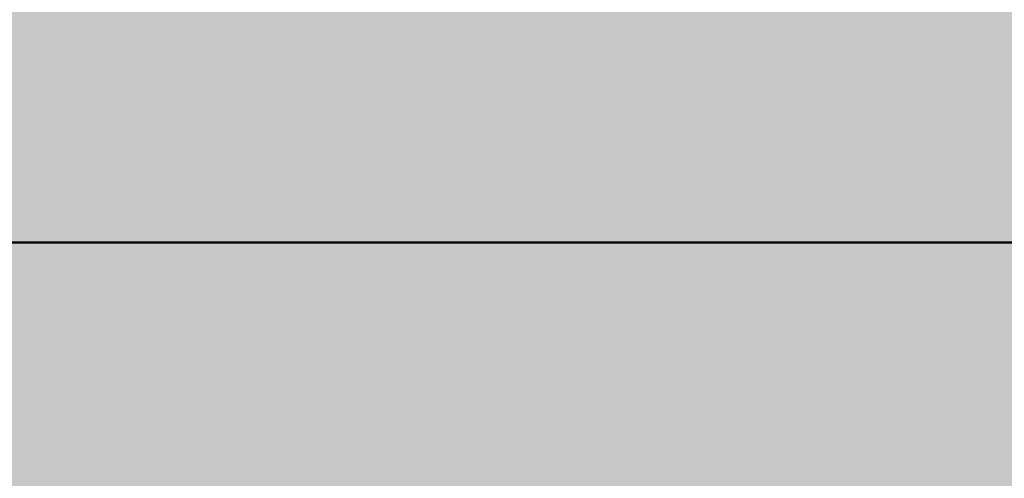
# Model space of a CAD drawing. Units: millimetres. Extents: x 0 to 2267, y 0 to 1823.
# Tile 142 of 256: x 1802 to 1823, y 1122 to 1132. Entities that reach past the tile are written whole.
import ezdxf

# ---------------------------------------------------------------- set-up
doc = ezdxf.new("R2010")
doc.units = ezdxf.units.MM
doc.header["$MEASUREMENT"] = 0
for name, color, linetype, lineweight in [('M-DIMS', 2, 'Continuous', 25), ('M-HATC', 252, 'Continuous', 18), ('M-OUTL', 7, 'Continuous', 50)]:
    doc.layers.add(name, color=color, linetype=linetype, lineweight=lineweight)
doc.styles.get("Standard").update_dxf_attribs({"font": 'arial.ttf'})
doc.dimstyles.get("Standard").update_dxf_attribs({"dimtxt": 7, "dimasz": 4, "dimexe": 0.18, "dimexo": 0.0625, "dimgap": 0.09, "dimtad": 0, "dimdec": 0, "dimzin": 0, "dimdsep": 46, "dimtxsty": 'Standard', "dimcen": 0.09, "dimadec": 0, "dimazin": 0, "dimtfac": 1, "dimtdec": 0, "dimtofl": 0, "dimtmove": 0, "dimatfit": 3, "dimfxl": 1, "dimtolj": 1, "dimtzin": 0, "dimarcsym": 0})

# ---------------------------------------------------------------- blocks, each defined once
blk = doc.blocks.new('*D1')
at = {"layer": 'Defpoints', "color": 0, "transparency": 16777216}
for p in [(1593.429, 1127.417), (1843.429, 1127.417), (1843.429, 955.628)]:
    blk.add_point(p, dxfattribs=at)
at = {"layer": 'M-DIMS', "color": 0, "lineweight": -2, "transparency": 16777216}
for p, q in [((1593.429, 1127.355), (1593.429, 955.448)), ((1843.429, 1127.355), (1843.429, 955.448)), ((1597.429, 955.628), (1710.558, 955.628)), ((1839.429, 955.628), (1726.3, 955.628))]:
    blk.add_line(p, q, dxfattribs=at)
at = {"layer": 'M-DIMS', "color": 0, "transparency": 16777216}
for points in [[(1597.429, 956.294), (1597.429, 954.961), (1593.429, 955.628)], [(1839.429, 956.294), (1839.429, 954.961), (1843.429, 955.628)]]:
    blk.add_solid(points, dxfattribs=at)
at = {"layer": 'M-DIMS', "color": 0, "transparency": 16777216, "insert": (1718.429, 955.628), "char_height": 7, "attachment_point": 5}
blk.add_mtext('\\A1;250', dxfattribs=at)

msp = doc.modelspace()

# ---------------------------------------------------------------- hatches: boundary and pattern name
at = {"layer": 'M-HATC'}
h = msp.add_hatch(color=256, dxfattribs=at)
h.dxf.hatch_style = 1
h.paths.add_polyline_path([(2055.771, 1603.062), (1381.087, 1603.062), (1381.087, 1598.062), (2055.771, 1598.062)])
h.paths.add_polyline_path([(2055.771, 1598.062), (1381.087, 1598.062), (1381.087, 1593.062), (2055.771, 1593.062)])
h.paths.add_polyline_path([(2051.307, 1536.761), (1385.55, 1536.761), (1385.55, 1526.761), (1387.55, 1526.761), (1388.537, 1525.053), (1385.332, 1521.233), (1385.332, 1521.223), (2050.254, 1522.749), (2048.321, 1525.053), (2049.307, 1526.761), (2051.307, 1526.761)])
edge = h.paths.add_edge_path()
edge.add_arc((1847.535, 1379.149), 135, 222.60306, 222.89085, ccw=False)
edge.add_line((1748.166, 1287.766), (1683.092, 1287.766))
edge.add_arc((1583.724, 1379.149), 135, 317.10915, 317.39694, ccw=False)
edge.add_arc((1678.969, 1290.671), 5, 222.8909, 317.1091, ccw=False)
edge.add_arc((1774.213, 1379.149), 135, 222.60306, 222.89085, ccw=False)
edge.add_line((1674.845, 1287.766), (1609.771, 1287.766))
edge.add_arc((1510.403, 1379.149), 135, 317.10915, 317.39694, ccw=False)
edge.add_arc((1605.647, 1290.671), 5, 222.8909, 317.1091, ccw=False)
edge.add_arc((1700.892, 1379.149), 135, 222.60306, 222.89085, ccw=False)
edge.add_line((1601.524, 1287.766), (1536.45, 1287.766))
edge.add_arc((1437.081, 1379.149), 135, 317.10915, 317.39694, ccw=False)
edge.add_arc((1532.326, 1290.671), 5, 222.8909, 317.1091, ccw=False)
edge.add_arc((1627.571, 1379.149), 135, 222.60306, 222.89085, ccw=False)
edge.add_line((1528.203, 1287.766), (1505.929, 1287.766))
edge.add_spline(control_points=[(1505.929, 1287.766), (1504.262, 1287.766), (1504.262, 1282.766), (1505.929, 1282.766)], knot_values=[0, 0, 0, 0, 5, 5, 5, 5], degree=3, periodic=0)
edge.add_line((1505.929, 1282.766), (1930.929, 1282.766))
edge.add_spline(control_points=[(1930.929, 1282.766), (1932.596, 1282.766), (1932.596, 1287.766), (1930.929, 1287.766)], knot_values=[0, 0, 0, 0, 5, 5, 5, 5], degree=3, periodic=0)
edge.add_line((1930.929, 1287.766), (1903.056, 1287.766))
edge.add_arc((1803.688, 1379.149), 135, 317.10915, 317.39694, ccw=False)
edge.add_arc((1898.932, 1290.671), 5, 222.8909, 317.1091, ccw=False)
edge.add_arc((1994.177, 1379.149), 135, 222.60306, 222.89085, ccw=False)
edge.add_line((1894.809, 1287.766), (1829.735, 1287.766))
edge.add_arc((1730.366, 1379.149), 135, 317.10915, 317.39694, ccw=False)
edge.add_arc((1825.611, 1290.671), 5, 222.8909, 317.1091, ccw=False)
edge.add_arc((1920.856, 1379.149), 135, 222.60306, 222.89085, ccw=False)
edge.add_line((1821.487, 1287.766), (1756.413, 1287.766))
edge.add_arc((1657.045, 1379.149), 135, 317.10915, 317.39694, ccw=False)
edge.add_arc((1752.29, 1290.671), 5, 222.8909, 317.1091, ccw=False)
edge = h.paths.add_edge_path()
edge.add_spline(control_points=[(1843.429, 1227.247), (1845.096, 1227.247), (1845.096, 1232.247), (1843.429, 1232.247)], knot_values=[0, 0, 0, 0, 5, 5, 5, 5], degree=3, periodic=0)
edge.add_line((1843.429, 1232.247), (1593.429, 1232.247))
edge.add_spline(control_points=[(1593.429, 1232.247), (1591.762, 1232.247), (1591.762, 1227.247), (1593.429, 1227.247)], knot_values=[0, 0, 0, 0, 5, 5, 5, 5], degree=3, periodic=0)
edge.add_line((1593.429, 1227.247), (1843.429, 1227.247))
h.paths.add_polyline_path([(1905.929, 1127.417), (1530.929, 1127.417, 0.414214), (1520.929, 1117.417), (1530.929, 1117.417), (1915.929, 1117.417, 0.414214)])
edge = h.paths.add_edge_path()
edge.add_arc((1397.086, 1498.408), 12.73, 90.7821, 190.8787, ccw=False)
edge.add_line((1396.912, 1511.136), (1428.01, 1511.349))
edge.add_line((1428.01, 1511.349), (1433.01, 1511.349))
edge.add_line((1433.01, 1511.349), (1434.439, 1511.349))
edge.add_arc((1419.474, 1498.08), 20, 41.561, 74.0821)
edge.add_line((1424.959, 1517.314), (1399.935, 1517.256))
edge.add_spline(control_points=[(1399.931, 1517.256), (1399.884, 1517.213), (1399.833, 1517.169), (1399.777, 1517.124)], knot_values=[11.567499, 11.567499, 11.567499, 11.567499, 11.814249, 11.814249, 11.814249, 11.814249], degree=3, periodic=0)
edge.add_spline(control_points=[(1399.633, 1517.01), (1399.583, 1516.972), (1399.531, 1516.934), (1399.476, 1516.895)], knot_values=[11.167718, 11.167718, 11.167718, 11.167718, 11.365188, 11.365188, 11.365188, 11.365188], degree=3, periodic=0)
edge.add_spline(control_points=[(1399.34, 1516.8), (1399.151, 1516.672), (1398.938, 1516.538), (1398.704, 1516.399)], knot_values=[10.376405, 10.376405, 10.376405, 10.376405, 11.00994, 11.00994, 11.00994, 11.00994], degree=3, periodic=0)
edge.add_spline(control_points=[(1398.657, 1516.372), (1398.579, 1516.326), (1398.498, 1516.28), (1398.415, 1516.233)], knot_values=[10.125175, 10.125175, 10.125175, 10.125175, 10.334406, 10.334406, 10.334406, 10.334406], degree=3, periodic=0)
edge.add_spline(control_points=[(1398.264, 1516.149), (1398.196, 1516.111), (1398.126, 1516.073), (1398.055, 1516.035)], knot_values=[9.832246, 9.832246, 9.832246, 9.832246, 9.999658, 9.999658, 9.999658, 9.999658], degree=3, periodic=0)
edge.add_spline(control_points=[(1397.999, 1516.005), (1397.731, 1515.862), (1397.446, 1515.717), (1397.147, 1515.571)], knot_values=[9.161808, 9.161808, 9.161808, 9.161808, 9.787769, 9.787769, 9.787769, 9.787769], degree=3, periodic=0)
edge.add_spline(control_points=[(1397.147, 1515.571), (1396.842, 1515.423), (1396.522, 1515.274), (1396.191, 1515.126)], knot_values=[8.524455, 8.524455, 8.524455, 8.524455, 9.161808, 9.161808, 9.161808, 9.161808], degree=3, periodic=0)
edge.add_spline(control_points=[(1396.078, 1515.076), (1395.985, 1515.035), (1395.892, 1514.994), (1395.798, 1514.953)], knot_values=[8.275193, 8.275193, 8.275193, 8.275193, 8.451726, 8.451726, 8.451726, 8.451726], degree=3, periodic=0)
edge.add_spline(control_points=[(1395.602, 1514.869), (1395.5, 1514.826), (1395.397, 1514.782), (1395.293, 1514.739)], knot_values=[7.962917, 7.962917, 7.962917, 7.962917, 8.152764, 8.152764, 8.152764, 8.152764], degree=3, periodic=0)
edge.add_spline(control_points=[(1395.212, 1514.706), (1394.828, 1514.547), (1394.435, 1514.393), (1394.036, 1514.244)], knot_values=[7.21254, 7.21254, 7.21254, 7.21254, 7.913148, 7.913148, 7.913148, 7.913148], degree=3, periodic=0)
edge.add_spline(control_points=[(1394.036, 1514.244), (1393.708, 1514.121), (1393.375, 1514.003), (1393.043, 1513.889)], knot_values=[6.633733, 6.633733, 6.633733, 6.633733, 7.21254, 7.21254, 7.21254, 7.21254], degree=3, periodic=0)
edge.add_spline(control_points=[(1392.821, 1513.815), (1392.72, 1513.781), (1392.618, 1513.748), (1392.517, 1513.715)], knot_values=[6.328796, 6.328796, 6.328796, 6.328796, 6.505493, 6.505493, 6.505493, 6.505493], degree=3, periodic=0)
edge.add_spline(control_points=[(1392.517, 1513.715), (1392.319, 1513.652), (1392.121, 1513.59), (1391.924, 1513.531)], knot_values=[5.984605, 5.984605, 5.984605, 5.984605, 6.328796, 6.328796, 6.328796, 6.328796], degree=3, periodic=0)
edge.add_spline(control_points=[(1391.792, 1513.491), (1391.312, 1513.35), (1390.838, 1513.224), (1390.378, 1513.117)], knot_values=[5.066697, 5.066697, 5.066697, 5.066697, 5.907055, 5.907055, 5.907055, 5.907055], degree=3, periodic=0)
edge.add_spline(control_points=[(1390.378, 1513.117), (1390.18, 1513.071), (1389.984, 1513.028), (1389.791, 1512.99)], knot_values=[4.70367, 4.70367, 4.70367, 4.70367, 5.066695, 5.066695, 5.066695, 5.066695], degree=3, periodic=0)
edge.add_spline(control_points=[(1389.422, 1512.92), (1389.246, 1512.889), (1389.073, 1512.862), (1388.904, 1512.838)], knot_values=[4.130571, 4.130571, 4.130571, 4.130571, 4.469816, 4.469816, 4.469816, 4.469816], degree=3, periodic=0)
edge.add_spline(control_points=[(1388.904, 1512.838), (1388.591, 1512.795), (1388.291, 1512.764), (1388.007, 1512.749)], knot_values=[3.504031, 3.504031, 3.504031, 3.504031, 4.130571, 4.130571, 4.130571, 4.130571], degree=3, periodic=0)
edge.add_spline(control_points=[(1387.936, 1512.746), (1387.854, 1512.742), (1387.773, 1512.74), (1387.694, 1512.739)], knot_values=[3.268866, 3.268866, 3.268866, 3.268866, 3.451164, 3.451164, 3.451164, 3.451164], degree=3, periodic=0)
edge.add_spline(control_points=[(1387.335, 1512.744), (1387.208, 1512.75), (1387.085, 1512.76), (1386.967, 1512.774)], knot_values=[2.670686, 2.670686, 2.670686, 2.670686, 2.984, 2.984, 2.984, 2.984], degree=3, periodic=0)
edge.add_spline(control_points=[(1386.833, 1512.792), (1386.821, 1512.794), (1386.809, 1512.796), (1386.797, 1512.798)], knot_values=[2.516981, 2.516981, 2.516981, 2.516981, 2.549528, 2.549528, 2.549528, 2.549528], degree=3, periodic=0)
edge.add_spline(control_points=[(1386.453, 1512.873), (1386.426, 1512.881), (1386.399, 1512.889), (1386.373, 1512.897)], knot_values=[2.095869, 2.095869, 2.095869, 2.095869, 2.17941, 2.17941, 2.17941, 2.17941], degree=3, periodic=0)
edge.add_spline(control_points=[(1386.069, 1513.019), (1386.063, 1513.022), (1386.058, 1513.025), (1386.052, 1513.028)], knot_values=[1.72453, 1.72453, 1.72453, 1.72453, 1.745933, 1.745933, 1.745933, 1.745933], degree=3, periodic=0)
edge.add_arc((1399.474, 1498.08), 20, 131.8243, 180)
edge.add_arc((1630.334, 1505.548), 250.971, 181.70518, 236.42798)
edge.add_arc((1605.34, 1483.304), 218.782, 238.66083, 243.34961)
edge.add_arc((1647.091, 1510.359), 262.899, 183.12984, 237.85344, ccw=False)
h.paths.add_polyline_path([(1406.537, 1391.964, 0.149382), (1491.551, 1296.442, -0.129517)], flags=17)
edge = h.paths.add_edge_path()
edge.add_arc((2037.384, 1498.08), 20, 0, 48.2659)
edge.add_spline(control_points=[(2050.697, 1513.005), (2050.651, 1512.985), (2050.603, 1512.966), (2050.554, 1512.948)], knot_values=[1.835652, 1.835652, 1.835652, 1.835652, 2.000781, 2.000781, 2.000781, 2.000781], degree=3, periodic=0)
edge.add_spline(control_points=[(2050.462, 1512.917), (2050.479, 1512.922), (2050.496, 1512.928), (2050.513, 1512.934)], knot_values=[2.045477, 2.045477, 2.045477, 2.045477, 2.101389, 2.101389, 2.101389, 2.101389], degree=3, periodic=0)
edge.add_spline(control_points=[(2050.129, 1512.834), (2050.198, 1512.847), (2050.266, 1512.862), (2050.331, 1512.879)], knot_values=[2.237629, 2.237629, 2.237629, 2.237629, 2.435841, 2.435841, 2.435841, 2.435841], degree=3, periodic=0)
edge.add_spline(control_points=[(2050.095, 1512.828), (2050.106, 1512.83), (2050.118, 1512.832), (2050.129, 1512.834)], knot_values=[2.435841, 2.435841, 2.435841, 2.435841, 2.468321, 2.468321, 2.468321, 2.468321], degree=3, periodic=0)
edge.add_spline(control_points=[(2049.784, 1512.785), (2049.855, 1512.792), (2049.924, 1512.801), (2049.992, 1512.811)], knot_values=[2.563852, 2.563852, 2.563852, 2.563852, 2.748541, 2.748541, 2.748541, 2.748541], degree=3, periodic=0)
edge.add_spline(control_points=[(2049.405, 1512.762), (2049.536, 1512.765), (2049.663, 1512.773), (2049.784, 1512.785)], knot_values=[2.748541, 2.748541, 2.748541, 2.748541, 3.064882, 3.064882, 3.064882, 3.064882], degree=3, periodic=0)
edge.add_spline(control_points=[(2049.17, 1512.76), (2049.234, 1512.759), (2049.297, 1512.759), (2049.358, 1512.761)], knot_values=[3.102309, 3.102309, 3.102309, 3.102309, 3.2503, 3.2503, 3.2503, 3.2503], degree=3, periodic=0)
edge.add_spline(control_points=[(2048.857, 1512.769), (2048.964, 1512.764), (2049.068, 1512.761), (2049.17, 1512.76)], knot_values=[3.2503, 3.2503, 3.2503, 3.2503, 3.486069, 3.486069, 3.486069, 3.486069], degree=3, periodic=0)
edge.add_spline(control_points=[(2048.692, 1512.779), (2048.373, 1512.801), (2048.035, 1512.841), (2047.682, 1512.897)], knot_values=[3.606429, 3.606429, 3.606429, 3.606429, 4.2989, 4.2989, 4.2989, 4.2989], degree=3, periodic=0)
edge.add_spline(control_points=[(2047.682, 1512.897), (2047.546, 1512.919), (2047.408, 1512.942), (2047.268, 1512.969)], knot_values=[4.2989, 4.2989, 4.2989, 4.2989, 4.565769, 4.565769, 4.565769, 4.565769], degree=3, periodic=0)
edge.add_spline(control_points=[(2047.268, 1512.969), (2047.145, 1512.991), (2047.021, 1513.016), (2046.895, 1513.042)], knot_values=[4.565769, 4.565769, 4.565769, 4.565769, 4.799971, 4.799971, 4.799971, 4.799971], degree=3, periodic=0)
edge.add_spline(control_points=[(2046.895, 1513.042), (2046.529, 1513.119), (2046.151, 1513.209), (2045.768, 1513.311)], knot_values=[4.799971, 4.799971, 4.799971, 4.799971, 5.483718, 5.483718, 5.483718, 5.483718], degree=3, periodic=0)
edge.add_spline(control_points=[(2045.768, 1513.311), (2045.372, 1513.415), (2044.97, 1513.532), (2044.566, 1513.659)], knot_values=[5.483718, 5.483718, 5.483718, 5.483718, 6.187866, 6.187866, 6.187866, 6.187866], degree=3, periodic=0)
edge.add_spline(control_points=[(2044.566, 1513.659), (2044.415, 1513.706), (2044.263, 1513.755), (2044.112, 1513.805)], knot_values=[6.187866, 6.187866, 6.187866, 6.187866, 6.451551, 6.451551, 6.451551, 6.451551], degree=3, periodic=0)
edge.add_spline(control_points=[(2044.112, 1513.805), (2043.997, 1513.843), (2043.882, 1513.881), (2043.767, 1513.92)], knot_values=[6.451551, 6.451551, 6.451551, 6.451551, 6.651434, 6.651434, 6.651434, 6.651434], degree=3, periodic=0)
edge.add_spline(control_points=[(2043.767, 1513.92), (2043.372, 1514.055), (2042.977, 1514.198), (2042.589, 1514.346)], knot_values=[6.651434, 6.651434, 6.651434, 6.651434, 7.338879, 7.338879, 7.338879, 7.338879], degree=3, periodic=0)
edge.add_spline(control_points=[(2042.589, 1514.346), (2042.164, 1514.507), (2041.746, 1514.675), (2041.341, 1514.846)], knot_values=[7.338879, 7.338879, 7.338879, 7.338879, 8.089209, 8.089209, 8.089209, 8.089209], degree=3, periodic=0)
edge.add_spline(control_points=[(2041.341, 1514.846), (2041.103, 1514.946), (2040.869, 1515.048), (2040.64, 1515.15)], knot_values=[8.089209, 8.089209, 8.089209, 8.089209, 8.529587, 8.529587, 8.529587, 8.529587], degree=3, periodic=0)
edge.add_spline(control_points=[(2040.51, 1515.209), (2040.082, 1515.402), (2039.675, 1515.597), (2039.295, 1515.789)], knot_values=[8.613818, 8.613818, 8.613818, 8.613818, 9.44571, 9.44571, 9.44571, 9.44571], degree=3, periodic=0)
edge.add_spline(control_points=[(2039.295, 1515.789), (2039.062, 1515.907), (2038.839, 1516.025), (2038.629, 1516.14)], knot_values=[9.44571, 9.44571, 9.44571, 9.44571, 9.956404, 9.956404, 9.956404, 9.956404], degree=3, periodic=0)
edge.add_spline(control_points=[(2038.629, 1516.14), (2038.519, 1516.2), (2038.412, 1516.26), (2038.309, 1516.319)], knot_values=[9.956404, 9.956404, 9.956404, 9.956404, 10.223542, 10.223542, 10.223542, 10.223542], degree=3, periodic=0)
edge.add_spline(control_points=[(2038.309, 1516.319), (2038.214, 1516.374), (2038.122, 1516.428), (2038.033, 1516.481)], knot_values=[10.223542, 10.223542, 10.223542, 10.223542, 10.47051, 10.47051, 10.47051, 10.47051], degree=3, periodic=0)
edge.add_spline(control_points=[(2038.033, 1516.481), (2037.786, 1516.63), (2037.564, 1516.773), (2037.372, 1516.909)], knot_values=[10.47051, 10.47051, 10.47051, 10.47051, 11.15767, 11.15767, 11.15767, 11.15767], degree=3, periodic=0)
edge.add_spline(control_points=[(2037.372, 1516.909), (2037.279, 1516.975), (2037.193, 1517.04), (2037.114, 1517.102)], knot_values=[11.15767, 11.15767, 11.15767, 11.15767, 11.49227, 11.49227, 11.49227, 11.49227], degree=3, periodic=0)
edge.add_spline(control_points=[(2036.856, 1517.326), (2036.915, 1517.269), (2036.981, 1517.21), (2037.056, 1517.149)], knot_values=[11.577341, 11.577341, 11.577341, 11.577341, 11.91035, 11.91035, 11.91035, 11.91035], degree=3, periodic=0)
edge.add_spline(control_points=[(2036.807, 1517.375), (2036.823, 1517.359), (2036.839, 1517.342), (2036.856, 1517.326)], knot_values=[11.91035, 11.91035, 11.91035, 11.91035, 12.007402, 12.007402, 12.007402, 12.007402], degree=3, periodic=0)
edge.add_spline(control_points=[(2036.702, 1517.494), (2036.71, 1517.483), (2036.72, 1517.472), (2036.729, 1517.461)], knot_values=[12.184155, 12.184155, 12.184155, 12.184155, 12.255409, 12.255409, 12.255409, 12.255409], degree=3, periodic=0)
edge.add_spline(control_points=[(2036.616, 1517.621), (2036.62, 1517.613), (2036.624, 1517.606), (2036.629, 1517.598)], knot_values=[12.487913, 12.487913, 12.487913, 12.487913, 12.541035, 12.541035, 12.541035, 12.541035], degree=3, periodic=0)
edge.add_spline(control_points=[(2036.563, 1517.786), (2036.564, 1517.779), (2036.564, 1517.773), (2036.565, 1517.766)], knot_values=[12.911761, 12.911761, 12.911761, 12.911761, 12.968286, 12.968286, 12.968286, 12.968286], degree=3, periodic=0)
edge.add_spline(control_points=[(2036.617, 1517.93), (2036.612, 1517.926), (2036.609, 1517.921), (2036.605, 1517.916)], knot_values=[13.382527, 13.382527, 13.382527, 13.382527, 13.433791, 13.433791, 13.433791, 13.433791], degree=3, periodic=0)
edge.add_spline(control_points=[(2036.749, 1518.017), (2036.736, 1518.012), (2036.724, 1518.006), (2036.712, 1518)], knot_values=[13.726299, 13.726299, 13.726299, 13.726299, 13.809928, 13.809928, 13.809928, 13.809928], degree=3, periodic=0)
edge.add_spline(control_points=[(2036.86, 1518.053), (2036.839, 1518.047), (2036.818, 1518.042), (2036.799, 1518.035)], knot_values=[13.910887, 13.910887, 13.910887, 13.910887, 14.02153, 14.02153, 14.02153, 14.02153], degree=3, periodic=0)
edge.add_line((2036.964, 1518.08), (2032.384, 1518.08))
edge.add_line((2032.384, 1518.08), (2027.384, 1518.08))
edge.add_line((2027.384, 1518.08), (2022.384, 1518.08))
edge.add_line((2022.384, 1518.08), (2017.384, 1518.08))
edge.add_arc((2017.384, 1498.08), 20, 90, 138.439)
edge.add_line((2002.419, 1511.349), (2003.848, 1511.349))
edge.add_line((2003.848, 1511.349), (2008.848, 1511.349))
edge.add_line((2008.848, 1511.349), (2039.772, 1511.138))
edge.add_arc((2039.772, 1498.408), 12.73, -10.8787, 90, ccw=False)
edge.add_arc((1789.767, 1510.359), 262.899, 302.14656, 356.87016, ccw=False)
edge.add_arc((1831.518, 1483.304), 218.782, 296.65039, 301.33917)
edge.add_arc((1806.524, 1505.548), 250.971, 303.57202, 358.29482)
h.paths.add_polyline_path([(2030.321, 1391.964, -0.129517), (1945.307, 1296.442, 0.149382)], flags=17)
edge = h.paths.add_edge_path()
edge.add_spline(control_points=[(2037.246, 1518.082), (2037.29, 1518.081), (2037.336, 1518.08), (2037.384, 1518.08)], knot_values=[0.000012, 0.000012, 0.000012, 0.000012, 0.144754, 0.144754, 0.144754, 0.144754], degree=3, periodic=0)
edge.add_line((2037.336, 1518.08), (2037.01, 1518.08))
edge.add_spline(control_points=[(2037.01, 1518.08), (2036.982, 1518.077), (2036.956, 1518.073), (2036.931, 1518.068)], knot_values=[14.13465, 14.13465, 14.13465, 14.13465, 14.247197, 14.247197, 14.247197, 14.247197], degree=3, periodic=0)
edge.add_spline(control_points=[(2036.931, 1518.068), (2036.928, 1518.067), (2036.924, 1518.067), (2036.921, 1518.066)], knot_values=[14.118315, 14.118315, 14.118315, 14.118315, 14.13465, 14.13465, 14.13465, 14.13465], degree=3, periodic=0)
edge.add_spline(control_points=[(2036.921, 1518.066), (2036.912, 1518.064), (2036.903, 1518.063), (2036.895, 1518.061)], knot_values=[14.078086, 14.078086, 14.078086, 14.078086, 14.118315, 14.118315, 14.118315, 14.118315], degree=3, periodic=0)
edge.add_spline(control_points=[(2036.895, 1518.061), (2036.883, 1518.058), (2036.872, 1518.056), (2036.86, 1518.053)], knot_values=[14.02153, 14.02153, 14.02153, 14.02153, 14.078086, 14.078086, 14.078086, 14.078086], degree=3, periodic=0)
edge.add_spline(control_points=[(2036.86, 1518.053), (2036.839, 1518.047), (2036.818, 1518.042), (2036.799, 1518.035)], knot_values=[13.910887, 13.910887, 13.910887, 13.910887, 14.02153, 14.02153, 14.02153, 14.02153], degree=3, periodic=0)
edge.add_spline(control_points=[(2036.799, 1518.035), (2036.798, 1518.035), (2036.797, 1518.035), (2036.797, 1518.035)], knot_values=[13.906906, 13.906906, 13.906906, 13.906906, 13.910887, 13.910887, 13.910887, 13.910887], degree=3, periodic=0)
edge.add_spline(control_points=[(2036.797, 1518.035), (2036.788, 1518.032), (2036.78, 1518.029), (2036.772, 1518.026)], knot_values=[13.857826, 13.857826, 13.857826, 13.857826, 13.906906, 13.906906, 13.906906, 13.906906], degree=3, periodic=0)
edge.add_spline(control_points=[(2036.772, 1518.026), (2036.764, 1518.023), (2036.756, 1518.02), (2036.749, 1518.017)], knot_values=[13.809928, 13.809928, 13.809928, 13.809928, 13.857826, 13.857826, 13.857826, 13.857826], degree=3, periodic=0)
edge.add_spline(control_points=[(2036.749, 1518.017), (2036.736, 1518.012), (2036.724, 1518.006), (2036.712, 1518)], knot_values=[13.726299, 13.726299, 13.726299, 13.726299, 13.809928, 13.809928, 13.809928, 13.809928], degree=3, periodic=0)
edge.add_spline(control_points=[(2036.712, 1518), (2036.712, 1518), (2036.712, 1518), (2036.711, 1518)], knot_values=[13.723993, 13.723993, 13.723993, 13.723993, 13.726299, 13.726299, 13.726299, 13.726299], degree=3, periodic=0)
edge.add_spline(control_points=[(2036.711, 1518), (2036.706, 1517.997), (2036.701, 1517.994), (2036.696, 1517.992)], knot_values=[13.686536, 13.686536, 13.686536, 13.686536, 13.723993, 13.723993, 13.723993, 13.723993], degree=3, periodic=0)
edge.add_spline(control_points=[(2036.696, 1517.992), (2036.692, 1517.989), (2036.687, 1517.987), (2036.683, 1517.984)], knot_values=[13.651251, 13.651251, 13.651251, 13.651251, 13.686536, 13.686536, 13.686536, 13.686536], degree=3, periodic=0)
edge.add_spline(control_points=[(2036.683, 1517.984), (2036.676, 1517.98), (2036.67, 1517.976), (2036.664, 1517.971)], knot_values=[13.596804, 13.596804, 13.596804, 13.596804, 13.651251, 13.651251, 13.651251, 13.651251], degree=3, periodic=0)
edge.add_spline(control_points=[(2036.664, 1517.971), (2036.664, 1517.971), (2036.663, 1517.971), (2036.663, 1517.971)], knot_values=[13.593956, 13.593956, 13.593956, 13.593956, 13.596804, 13.596804, 13.596804, 13.596804], degree=3, periodic=0)
edge.add_spline(control_points=[(2036.663, 1517.971), (2036.66, 1517.969), (2036.658, 1517.967), (2036.655, 1517.965)], knot_values=[13.570322, 13.570322, 13.570322, 13.570322, 13.593956, 13.593956, 13.593956, 13.593956], degree=3, periodic=0)
edge.add_spline(control_points=[(2036.655, 1517.965), (2036.653, 1517.963), (2036.65, 1517.961), (2036.647, 1517.959)], knot_values=[13.545477, 13.545477, 13.545477, 13.545477, 13.570322, 13.570322, 13.570322, 13.570322], degree=3, periodic=0)
edge.add_spline(control_points=[(2036.647, 1517.959), (2036.647, 1517.959), (2036.647, 1517.959), (2036.647, 1517.959)], knot_values=[13.543931, 13.543931, 13.543931, 13.543931, 13.545477, 13.545477, 13.545477, 13.545477], degree=3, periodic=0)
edge.add_spline(control_points=[(2036.647, 1517.959), (2036.641, 1517.954), (2036.636, 1517.949), (2036.631, 1517.945)], knot_values=[13.488237, 13.488237, 13.488237, 13.488237, 13.543931, 13.543931, 13.543931, 13.543931], degree=3, periodic=0)
edge.add_spline(control_points=[(2036.631, 1517.945), (2036.628, 1517.942), (2036.626, 1517.94), (2036.623, 1517.937)], knot_values=[13.460307, 13.460307, 13.460307, 13.460307, 13.488237, 13.488237, 13.488237, 13.488237], degree=3, periodic=0)
edge.add_spline(control_points=[(2036.623, 1517.937), (2036.622, 1517.936), (2036.62, 1517.934), (2036.618, 1517.932)], knot_values=[13.439712, 13.439712, 13.439712, 13.439712, 13.460307, 13.460307, 13.460307, 13.460307], degree=3, periodic=0)
edge.add_spline(control_points=[(2036.618, 1517.932), (2036.618, 1517.931), (2036.617, 1517.931), (2036.617, 1517.93)], knot_values=[13.433791, 13.433791, 13.433791, 13.433791, 13.439712, 13.439712, 13.439712, 13.439712], degree=3, periodic=0)
edge.add_spline(control_points=[(2036.617, 1517.93), (2036.612, 1517.926), (2036.609, 1517.921), (2036.605, 1517.916)], knot_values=[13.382527, 13.382527, 13.382527, 13.382527, 13.433791, 13.433791, 13.433791, 13.433791], degree=3, periodic=0)
edge.add_spline(control_points=[(2036.605, 1517.916), (2036.603, 1517.913), (2036.6, 1517.91), (2036.598, 1517.907)], knot_values=[13.350017, 13.350017, 13.350017, 13.350017, 13.382527, 13.382527, 13.382527, 13.382527], degree=3, periodic=0)
edge.add_spline(control_points=[(2036.598, 1517.907), (2036.597, 1517.906), (2036.596, 1517.904), (2036.595, 1517.903)], knot_values=[13.333922, 13.333922, 13.333922, 13.333922, 13.350017, 13.350017, 13.350017, 13.350017], degree=3, periodic=0)
edge.add_spline(control_points=[(2036.595, 1517.903), (2036.595, 1517.902), (2036.594, 1517.901), (2036.593, 1517.9)], knot_values=[13.323828, 13.323828, 13.323828, 13.323828, 13.333922, 13.333922, 13.333922, 13.333922], degree=3, periodic=0)
edge.add_spline(control_points=[(2036.593, 1517.9), (2036.59, 1517.895), (2036.588, 1517.891), (2036.585, 1517.886)], knot_values=[13.277545, 13.277545, 13.277545, 13.277545, 13.323828, 13.323828, 13.323828, 13.323828], degree=3, periodic=0)
edge.add_spline(control_points=[(2036.585, 1517.886), (2036.584, 1517.883), (2036.582, 1517.879), (2036.58, 1517.875)], knot_values=[13.240119, 13.240119, 13.240119, 13.240119, 13.277545, 13.277545, 13.277545, 13.277545], degree=3, periodic=0)
edge.add_spline(control_points=[(2036.58, 1517.875), (2036.58, 1517.874), (2036.579, 1517.873), (2036.578, 1517.872)], knot_values=[13.228211, 13.228211, 13.228211, 13.228211, 13.240119, 13.240119, 13.240119, 13.240119], degree=3, periodic=0)
edge.add_spline(control_points=[(2036.578, 1517.872), (2036.578, 1517.87), (2036.577, 1517.869), (2036.577, 1517.868)], knot_values=[13.215717, 13.215717, 13.215717, 13.215717, 13.228211, 13.228211, 13.228211, 13.228211], degree=3, periodic=0)
edge.add_spline(control_points=[(2036.577, 1517.868), (2036.575, 1517.864), (2036.574, 1517.86), (2036.573, 1517.857)], knot_values=[13.179847, 13.179847, 13.179847, 13.179847, 13.215717, 13.215717, 13.215717, 13.215717], degree=3, periodic=0)
edge.add_spline(control_points=[(2036.573, 1517.857), (2036.571, 1517.851), (2036.57, 1517.846), (2036.569, 1517.841)], knot_values=[13.132017, 13.132017, 13.132017, 13.132017, 13.179847, 13.179847, 13.179847, 13.179847], degree=3, periodic=0)
edge.add_spline(control_points=[(2036.569, 1517.841), (2036.568, 1517.84), (2036.568, 1517.839), (2036.568, 1517.838)], knot_values=[13.122482, 13.122482, 13.122482, 13.122482, 13.132017, 13.132017, 13.132017, 13.132017], degree=3, periodic=0)
edge.add_spline(control_points=[(2036.568, 1517.838), (2036.568, 1517.836), (2036.567, 1517.835), (2036.567, 1517.833)], knot_values=[13.105592, 13.105592, 13.105592, 13.105592, 13.122482, 13.122482, 13.122482, 13.122482], degree=3, periodic=0)
edge.add_spline(control_points=[(2036.567, 1517.833), (2036.566, 1517.829), (2036.566, 1517.826), (2036.565, 1517.822)], knot_values=[13.074063, 13.074063, 13.074063, 13.074063, 13.105592, 13.105592, 13.105592, 13.105592], degree=3, periodic=0)
edge.add_spline(control_points=[(2036.565, 1517.822), (2036.565, 1517.822), (2036.565, 1517.822), (2036.565, 1517.822)], knot_values=[13.074043, 13.074043, 13.074043, 13.074043, 13.074063, 13.074063, 13.074063, 13.074063], degree=3, periodic=0)
edge.add_spline(control_points=[(2036.565, 1517.822), (2036.564, 1517.816), (2036.564, 1517.811), (2036.564, 1517.805)], knot_values=[13.021884, 13.021884, 13.021884, 13.021884, 13.074043, 13.074043, 13.074043, 13.074043], degree=3, periodic=0)
edge.add_spline(control_points=[(2036.564, 1517.805), (2036.564, 1517.804), (2036.564, 1517.803), (2036.564, 1517.803)], knot_values=[13.01674, 13.01674, 13.01674, 13.01674, 13.021884, 13.021884, 13.021884, 13.021884], degree=3, periodic=0)
edge.add_spline(control_points=[(2036.564, 1517.803), (2036.563, 1517.801), (2036.563, 1517.798), (2036.563, 1517.796)], knot_values=[12.996438, 12.996438, 12.996438, 12.996438, 13.01674, 13.01674, 13.01674, 13.01674], degree=3, periodic=0)
edge.add_spline(control_points=[(2036.563, 1517.796), (2036.563, 1517.793), (2036.563, 1517.789), (2036.563, 1517.786)], knot_values=[12.968286, 12.968286, 12.968286, 12.968286, 12.996438, 12.996438, 12.996438, 12.996438], degree=3, periodic=0)
edge.add_spline(control_points=[(2036.563, 1517.786), (2036.564, 1517.779), (2036.564, 1517.773), (2036.565, 1517.766)], knot_values=[12.911761, 12.911761, 12.911761, 12.911761, 12.968286, 12.968286, 12.968286, 12.968286], degree=3, periodic=0)
edge.add_spline(control_points=[(2036.565, 1517.766), (2036.565, 1517.766), (2036.565, 1517.766), (2036.565, 1517.766)], knot_values=[12.911017, 12.911017, 12.911017, 12.911017, 12.911761, 12.911761, 12.911761, 12.911761], degree=3, periodic=0)
edge.add_spline(control_points=[(2036.565, 1517.766), (2036.565, 1517.762), (2036.566, 1517.759), (2036.566, 1517.756)], knot_values=[12.88528, 12.88528, 12.88528, 12.88528, 12.911017, 12.911017, 12.911017, 12.911017], degree=3, periodic=0)
edge.add_spline(control_points=[(2036.566, 1517.756), (2036.567, 1517.753), (2036.567, 1517.751), (2036.568, 1517.748)], knot_values=[12.862519, 12.862519, 12.862519, 12.862519, 12.88528, 12.88528, 12.88528, 12.88528], degree=3, periodic=0)
edge.add_spline(control_points=[(2036.568, 1517.748), (2036.568, 1517.747), (2036.568, 1517.747), (2036.568, 1517.746)], knot_values=[12.858885, 12.858885, 12.858885, 12.858885, 12.862519, 12.862519, 12.862519, 12.862519], degree=3, periodic=0)
edge.add_spline(control_points=[(2036.568, 1517.746), (2036.569, 1517.74), (2036.571, 1517.733), (2036.572, 1517.726)], knot_values=[12.8053, 12.8053, 12.8053, 12.8053, 12.858885, 12.858885, 12.858885, 12.858885], degree=3, periodic=0)
edge.add_spline(control_points=[(2036.572, 1517.726), (2036.573, 1517.723), (2036.574, 1517.719), (2036.576, 1517.715)], knot_values=[12.775176, 12.775176, 12.775176, 12.775176, 12.8053, 12.8053, 12.8053, 12.8053], degree=3, periodic=0)
edge.add_spline(control_points=[(2036.576, 1517.715), (2036.576, 1517.713), (2036.577, 1517.71), (2036.578, 1517.708)], knot_values=[12.756759, 12.756759, 12.756759, 12.756759, 12.775176, 12.775176, 12.775176, 12.775176], degree=3, periodic=0)
edge.add_spline(control_points=[(2036.578, 1517.708), (2036.578, 1517.707), (2036.578, 1517.706), (2036.579, 1517.705)], knot_values=[12.748742, 12.748742, 12.748742, 12.748742, 12.756759, 12.756759, 12.756759, 12.756759], degree=3, periodic=0)
edge.add_spline(control_points=[(2036.579, 1517.705), (2036.581, 1517.698), (2036.583, 1517.692), (2036.586, 1517.685)], knot_values=[12.69959, 12.69959, 12.69959, 12.69959, 12.748742, 12.748742, 12.748742, 12.748742], degree=3, periodic=0)
edge.add_spline(control_points=[(2036.586, 1517.685), (2036.588, 1517.68), (2036.59, 1517.675), (2036.592, 1517.669)], knot_values=[12.659038, 12.659038, 12.659038, 12.659038, 12.69959, 12.69959, 12.69959, 12.69959], degree=3, periodic=0)
edge.add_spline(control_points=[(2036.592, 1517.669), (2036.594, 1517.665), (2036.596, 1517.66), (2036.598, 1517.656)], knot_values=[12.626806, 12.626806, 12.626806, 12.626806, 12.659038, 12.659038, 12.659038, 12.659038], degree=3, periodic=0)
edge.add_spline(control_points=[(2036.598, 1517.656), (2036.598, 1517.655), (2036.599, 1517.654), (2036.599, 1517.653)], knot_values=[12.619394, 12.619394, 12.619394, 12.619394, 12.626806, 12.626806, 12.626806, 12.626806], degree=3, periodic=0)
edge.add_spline(control_points=[(2036.599, 1517.653), (2036.604, 1517.642), (2036.61, 1517.632), (2036.616, 1517.621)], knot_values=[12.541039, 12.541039, 12.541039, 12.541039, 12.619394, 12.619394, 12.619394, 12.619394], degree=3, periodic=0)
edge.add_spline(control_points=[(2036.616, 1517.621), (2036.616, 1517.621), (2036.616, 1517.621), (2036.616, 1517.621)], knot_values=[12.541035, 12.541035, 12.541035, 12.541035, 12.541039, 12.541039, 12.541039, 12.541039], degree=3, periodic=0)
edge.add_spline(control_points=[(2036.616, 1517.621), (2036.62, 1517.613), (2036.624, 1517.606), (2036.629, 1517.598)], knot_values=[12.487913, 12.487913, 12.487913, 12.487913, 12.541035, 12.541035, 12.541035, 12.541035], degree=3, periodic=0)
edge.add_spline(control_points=[(2036.629, 1517.598), (2036.633, 1517.592), (2036.637, 1517.585), (2036.641, 1517.579)], knot_values=[12.443982, 12.443982, 12.443982, 12.443982, 12.487913, 12.487913, 12.487913, 12.487913], degree=3, periodic=0)
edge.add_spline(control_points=[(2036.641, 1517.579), (2036.641, 1517.578), (2036.642, 1517.576), (2036.643, 1517.575)], knot_values=[12.434996, 12.434996, 12.434996, 12.434996, 12.443982, 12.443982, 12.443982, 12.443982], degree=3, periodic=0)
edge.add_spline(control_points=[(2036.643, 1517.575), (2036.653, 1517.56), (2036.664, 1517.544), (2036.676, 1517.528)], knot_values=[12.329647, 12.329647, 12.329647, 12.329647, 12.434996, 12.434996, 12.434996, 12.434996], degree=3, periodic=0)
edge.add_spline(control_points=[(2036.676, 1517.528), (2036.684, 1517.517), (2036.693, 1517.505), (2036.702, 1517.494)], knot_values=[12.255409, 12.255409, 12.255409, 12.255409, 12.329647, 12.329647, 12.329647, 12.329647], degree=3, periodic=0)
edge.add_spline(control_points=[(2036.702, 1517.494), (2036.71, 1517.483), (2036.72, 1517.472), (2036.729, 1517.461)], knot_values=[12.184155, 12.184155, 12.184155, 12.184155, 12.255409, 12.255409, 12.255409, 12.255409], degree=3, periodic=0)
edge.add_spline(control_points=[(2036.729, 1517.461), (2036.744, 1517.444), (2036.759, 1517.426), (2036.775, 1517.409)], knot_values=[12.075961, 12.075961, 12.075961, 12.075961, 12.184155, 12.184155, 12.184155, 12.184155], degree=3, periodic=0)
edge.add_spline(control_points=[(2036.775, 1517.409), (2036.776, 1517.407), (2036.777, 1517.406), (2036.778, 1517.405)], knot_values=[12.069502, 12.069502, 12.069502, 12.069502, 12.075961, 12.075961, 12.075961, 12.075961], degree=3, periodic=0)
edge.add_spline(control_points=[(2036.778, 1517.405), (2036.788, 1517.395), (2036.797, 1517.385), (2036.807, 1517.375)], knot_values=[12.007402, 12.007402, 12.007402, 12.007402, 12.069502, 12.069502, 12.069502, 12.069502], degree=3, periodic=0)
edge.add_spline(control_points=[(2036.807, 1517.375), (2036.823, 1517.359), (2036.839, 1517.342), (2036.856, 1517.326)], knot_values=[11.91035, 11.91035, 11.91035, 11.91035, 12.007402, 12.007402, 12.007402, 12.007402], degree=3, periodic=0)
edge.add_spline(control_points=[(2036.856, 1517.326), (2036.915, 1517.269), (2036.981, 1517.21), (2037.056, 1517.149)], knot_values=[11.577341, 11.577341, 11.577341, 11.577341, 11.91035, 11.91035, 11.91035, 11.91035], degree=3, periodic=0)
edge.add_spline(control_points=[(2037.056, 1517.149), (2037.075, 1517.134), (2037.094, 1517.118), (2037.114, 1517.102)], knot_values=[11.49227, 11.49227, 11.49227, 11.49227, 11.577341, 11.577341, 11.577341, 11.577341], degree=3, periodic=0)
edge.add_spline(control_points=[(2037.114, 1517.102), (2037.193, 1517.04), (2037.279, 1516.975), (2037.372, 1516.909)], knot_values=[11.15767, 11.15767, 11.15767, 11.15767, 11.49227, 11.49227, 11.49227, 11.49227], degree=3, periodic=0)
edge.add_spline(control_points=[(2037.372, 1516.909), (2037.564, 1516.773), (2037.786, 1516.63), (2038.033, 1516.481)], knot_values=[10.47051, 10.47051, 10.47051, 10.47051, 11.15767, 11.15767, 11.15767, 11.15767], degree=3, periodic=0)
edge.add_spline(control_points=[(2038.033, 1516.481), (2038.122, 1516.428), (2038.214, 1516.374), (2038.309, 1516.319)], knot_values=[10.223542, 10.223542, 10.223542, 10.223542, 10.47051, 10.47051, 10.47051, 10.47051], degree=3, periodic=0)
edge.add_spline(control_points=[(2038.309, 1516.319), (2038.412, 1516.26), (2038.519, 1516.2), (2038.629, 1516.14)], knot_values=[9.956404, 9.956404, 9.956404, 9.956404, 10.223542, 10.223542, 10.223542, 10.223542], degree=3, periodic=0)
edge.add_spline(control_points=[(2038.629, 1516.14), (2038.839, 1516.025), (2039.062, 1515.907), (2039.295, 1515.789)], knot_values=[9.44571, 9.44571, 9.44571, 9.44571, 9.956404, 9.956404, 9.956404, 9.956404], degree=3, periodic=0)
edge.add_spline(control_points=[(2039.295, 1515.789), (2039.675, 1515.597), (2040.082, 1515.402), (2040.51, 1515.209)], knot_values=[8.613818, 8.613818, 8.613818, 8.613818, 9.44571, 9.44571, 9.44571, 9.44571], degree=3, periodic=0)
edge.add_spline(control_points=[(2040.51, 1515.209), (2040.553, 1515.189), (2040.597, 1515.17), (2040.64, 1515.15)], knot_values=[8.529587, 8.529587, 8.529587, 8.529587, 8.613818, 8.613818, 8.613818, 8.613818], degree=3, periodic=0)
edge.add_spline(control_points=[(2040.64, 1515.15), (2040.869, 1515.048), (2041.103, 1514.946), (2041.341, 1514.846)], knot_values=[8.089209, 8.089209, 8.089209, 8.089209, 8.529587, 8.529587, 8.529587, 8.529587], degree=3, periodic=0)
edge.add_spline(control_points=[(2041.341, 1514.846), (2041.746, 1514.675), (2042.164, 1514.507), (2042.589, 1514.346)], knot_values=[7.338879, 7.338879, 7.338879, 7.338879, 8.089209, 8.089209, 8.089209, 8.089209], degree=3, periodic=0)
edge.add_spline(control_points=[(2042.589, 1514.346), (2042.977, 1514.198), (2043.372, 1514.055), (2043.767, 1513.92)], knot_values=[6.651434, 6.651434, 6.651434, 6.651434, 7.338879, 7.338879, 7.338879, 7.338879], degree=3, periodic=0)
edge.add_spline(control_points=[(2043.767, 1513.92), (2043.882, 1513.881), (2043.997, 1513.843), (2044.112, 1513.805)], knot_values=[6.451551, 6.451551, 6.451551, 6.451551, 6.651434, 6.651434, 6.651434, 6.651434], degree=3, periodic=0)
edge.add_spline(control_points=[(2044.112, 1513.805), (2044.263, 1513.755), (2044.415, 1513.706), (2044.566, 1513.659)], knot_values=[6.187866, 6.187866, 6.187866, 6.187866, 6.451551, 6.451551, 6.451551, 6.451551], degree=3, periodic=0)
edge.add_spline(control_points=[(2044.566, 1513.659), (2044.97, 1513.532), (2045.372, 1513.415), (2045.768, 1513.311)], knot_values=[5.483718, 5.483718, 5.483718, 5.483718, 6.187866, 6.187866, 6.187866, 6.187866], degree=3, periodic=0)
edge.add_spline(control_points=[(2045.768, 1513.311), (2046.151, 1513.209), (2046.529, 1513.119), (2046.895, 1513.042)], knot_values=[4.799971, 4.799971, 4.799971, 4.799971, 5.483718, 5.483718, 5.483718, 5.483718], degree=3, periodic=0)
edge.add_spline(control_points=[(2046.895, 1513.042), (2047.021, 1513.016), (2047.145, 1512.991), (2047.268, 1512.969)], knot_values=[4.565769, 4.565769, 4.565769, 4.565769, 4.799971, 4.799971, 4.799971, 4.799971], degree=3, periodic=0)
edge.add_spline(control_points=[(2047.268, 1512.969), (2047.408, 1512.942), (2047.546, 1512.919), (2047.682, 1512.897)], knot_values=[4.2989, 4.2989, 4.2989, 4.2989, 4.565769, 4.565769, 4.565769, 4.565769], degree=3, periodic=0)
edge.add_spline(control_points=[(2047.682, 1512.897), (2048.035, 1512.841), (2048.373, 1512.801), (2048.692, 1512.779)], knot_values=[3.606429, 3.606429, 3.606429, 3.606429, 4.2989, 4.2989, 4.2989, 4.2989], degree=3, periodic=0)
edge.add_spline(control_points=[(2048.692, 1512.779), (2048.748, 1512.775), (2048.803, 1512.772), (2048.857, 1512.769)], knot_values=[3.486069, 3.486069, 3.486069, 3.486069, 3.606429, 3.606429, 3.606429, 3.606429], degree=3, periodic=0)
edge.add_spline(control_points=[(2048.857, 1512.769), (2048.964, 1512.764), (2049.068, 1512.761), (2049.17, 1512.76)], knot_values=[3.2503, 3.2503, 3.2503, 3.2503, 3.486069, 3.486069, 3.486069, 3.486069], degree=3, periodic=0)
edge.add_spline(control_points=[(2049.17, 1512.76), (2049.234, 1512.759), (2049.297, 1512.759), (2049.358, 1512.761)], knot_values=[3.102309, 3.102309, 3.102309, 3.102309, 3.2503, 3.2503, 3.2503, 3.2503], degree=3, periodic=0)
edge.add_spline(control_points=[(2049.358, 1512.761), (2049.374, 1512.761), (2049.39, 1512.761), (2049.405, 1512.762)], knot_values=[3.064882, 3.064882, 3.064882, 3.064882, 3.102309, 3.102309, 3.102309, 3.102309], degree=3, periodic=0)
edge.add_spline(control_points=[(2049.405, 1512.762), (2049.536, 1512.765), (2049.663, 1512.773), (2049.784, 1512.785)], knot_values=[2.748541, 2.748541, 2.748541, 2.748541, 3.064882, 3.064882, 3.064882, 3.064882], degree=3, periodic=0)
edge.add_spline(control_points=[(2049.784, 1512.785), (2049.855, 1512.792), (2049.924, 1512.801), (2049.992, 1512.811)], knot_values=[2.563852, 2.563852, 2.563852, 2.563852, 2.748541, 2.748541, 2.748541, 2.748541], degree=3, periodic=0)
edge.add_spline(control_points=[(2049.992, 1512.811), (2050.026, 1512.816), (2050.061, 1512.822), (2050.095, 1512.828)], knot_values=[2.468321, 2.468321, 2.468321, 2.468321, 2.563852, 2.563852, 2.563852, 2.563852], degree=3, periodic=0)
edge.add_spline(control_points=[(2050.095, 1512.828), (2050.106, 1512.83), (2050.118, 1512.832), (2050.129, 1512.834)], knot_values=[2.435841, 2.435841, 2.435841, 2.435841, 2.468321, 2.468321, 2.468321, 2.468321], degree=3, periodic=0)
edge.add_spline(control_points=[(2050.129, 1512.834), (2050.198, 1512.847), (2050.266, 1512.862), (2050.331, 1512.879)], knot_values=[2.237629, 2.237629, 2.237629, 2.237629, 2.435841, 2.435841, 2.435841, 2.435841], degree=3, periodic=0)
edge.add_spline(control_points=[(2050.331, 1512.879), (2050.375, 1512.891), (2050.419, 1512.903), (2050.462, 1512.917)], knot_values=[2.101389, 2.101389, 2.101389, 2.101389, 2.237629, 2.237629, 2.237629, 2.237629], degree=3, periodic=0)
edge.add_spline(control_points=[(2050.462, 1512.917), (2050.479, 1512.922), (2050.496, 1512.928), (2050.513, 1512.934)], knot_values=[2.045477, 2.045477, 2.045477, 2.045477, 2.101389, 2.101389, 2.101389, 2.101389], degree=3, periodic=0)
edge.add_spline(control_points=[(2050.513, 1512.934), (2050.527, 1512.938), (2050.54, 1512.943), (2050.554, 1512.948)], knot_values=[2.000781, 2.000781, 2.000781, 2.000781, 2.045477, 2.045477, 2.045477, 2.045477], degree=3, periodic=0)
edge.add_spline(control_points=[(2050.554, 1512.948), (2050.603, 1512.966), (2050.651, 1512.985), (2050.697, 1513.005)], knot_values=[1.835652, 1.835652, 1.835652, 1.835652, 2.000781, 2.000781, 2.000781, 2.000781], degree=3, periodic=0)
edge.add_arc((2037.384, 1498.08), 20, 48.2659, 90.1299)
edge = h.paths.add_edge_path(flags=16)
edge.add_spline(control_points=[(1386.139, 1512.986), (1388.92, 1511.739), (1398.039, 1515.519), (1399.931, 1517.256)], knot_values=[1.831046, 1.831046, 1.831046, 1.831046, 11.814249, 11.814249, 11.814249, 11.814249], degree=3, periodic=0)
edge.add_line((1399.931, 1517.256), (1393.743, 1517.242))
edge.add_arc((1399.474, 1498.08), 20, 106.6501, 131.8173)
h = msp.add_hatch(color=256, dxfattribs=at)
h.dxf.hatch_style = 1
h.paths.add_polyline_path([(2042.889, 1580.18), (2055.771, 1593.062), (1381.087, 1593.062), (1393.969, 1580.18), (1374.086, 1560.296), (2062.772, 1560.296)])
h.paths.add_polyline_path([(1843.429, 1201.33), (1843.429, 1227.247), (1593.429, 1227.247), (1593.429, 1201.33, -0.228274), (1574.599, 1162.235), (1530.929, 1127.417), (1905.929, 1127.417), (1862.259, 1162.235, -0.228274)])

# ---------------------------------------------------------------- linework, layer by layer
at = {"layer": 'M-OUTL'}
msp.add_line((1530.929, 1127.417), (1905.929, 1127.417), dxfattribs=at)

# ---------------------------------------------------------------- dimensions: what is measured, and where the dimension line sits
at = {"layer": 'M-DIMS'}
dim = msp.add_linear_dim(base=(1843.429, 955.628), p1=(1593.429, 1127.417), p2=(1843.429, 1127.417), dimstyle='Standard', override={"dimclrd": 0, "dimclre": 0, "dimclrt": 0}, dxfattribs=at)
dim.commit()
dim.dimension.update_dxf_attribs({"geometry": '*D1', "text_midpoint": (1718.429, 955.628)})

doc.saveas('drawing.dxf')
